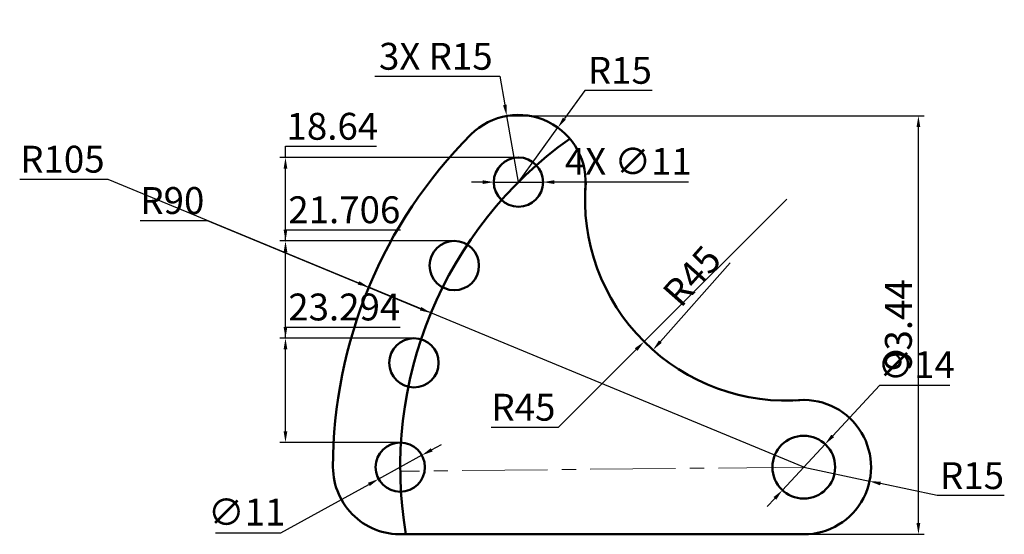
# Model space of a CAD drawing. Units: millimetres. Extents: x 68 to 288, y 29 to 144.
import ezdxf

# ---------------------------------------------------------------- set-up
doc = ezdxf.new("R2010")
doc.units = ezdxf.units.MM
doc.linetypes.add('CENTER2', pattern=[28.575, 19.05, -3.175, 3.175, -3.175])
for name, color, linetype, lineweight in [('M-CNTR', 4, 'CENTER2', 18), ('M-DIMS', 2, 'Continuous', 25), ('M-OUTL', 7, 'Continuous', 50)]:
    doc.layers.add(name, color=color, linetype=linetype, lineweight=lineweight)
doc.styles.get("Standard").update_dxf_attribs({"font": 'arial.ttf'})
doc.dimstyles.new('ISO-25', dxfattribs={"dimtxt": 6, "dimasz": 2.5, "dimexe": 1.25, "dimexo": 0.625, "dimtad": 1, "dimtoh": 1, "dimdec": 0, "dimtxsty": 'Standard', "dimcen": 2.5, "dimadec": 0, "dimazin": 0, "dimtfac": 1, "dimtdec": 0, "dimtmove": 0, "dimatfit": 3, "dimfxl": 1, "dimarcsym": 0})

# ---------------------------------------------------------------- blocks, each defined once
blk = doc.blocks.new('*U1')
blk.add_circle((0, 0), 5.5)
blk = doc.blocks.new('*U2')
at = {"layer": 'M-OUTL', "color": 0, "linetype": 'ByBlock', "lineweight": -2, "transparency": 16777216}
for p, rotation in [((49.87, 107.45), 315.0000000000001), ((35.56, 88.81), 330.0000000000001), ((26.57, 67.1), 344.9999999999999)]:
    blk.add_blockref('*U1', p, dxfattribs=dict(at, rotation=rotation))
blk.add_blockref('*U1', (23.51, 43.81), dxfattribs=at)
blk = doc.blocks.new('*D3')
at = {"layer": 'Defpoints', "color": 0, "transparency": 16777216}
for p in [(239.43, 103.65), (209.58, 69.97)]:
    blk.add_point(p, dxfattribs=at)
at = {"layer": 'M-DIMS', "color": 0, "lineweight": -2, "transparency": 16777216}
blk.add_line((226.8, 89.4), (211.24, 71.84), dxfattribs=at)
at = {"layer": 'M-DIMS', "color": 0, "transparency": 16777216}
blk.add_solid([(210.93, 72.11), (211.55, 71.56), (209.58, 69.97)], dxfattribs=at)
at = {"layer": 'M-DIMS', "color": 0, "transparency": 16777216, "insert": (218.86, 85.98), "char_height": 6, "attachment_point": 5, "rotation": 48.4597}
blk.add_mtext('R45', dxfattribs=at)
blk = doc.blocks.new('*D4')
at = {"layer": 'Defpoints', "color": 0, "transparency": 16777216}
for p in [(247.98, 48.95), (238.47, 38.67)]:
    blk.add_point(p, dxfattribs=at)
at = {"layer": 'M-DIMS', "color": 0, "lineweight": -2, "transparency": 16777216}
for p, q in [((260.11, 62.06), (249.68, 50.78)), ((275.84, 62.06), (260.11, 62.06)), ((238.47, 38.67), (247.98, 48.95)), ((236.77, 36.84), (235.08, 35))]:
    blk.add_line(p, q, dxfattribs=at)
at = {"layer": 'M-DIMS', "color": 0, "transparency": 16777216}
for points in [[(249.37, 51.06), (249.98, 50.5), (247.98, 48.95)], [(236.47, 37.12), (237.08, 36.55), (238.47, 38.67)]]:
    blk.add_solid(points, dxfattribs=at)
at = {"layer": 'M-DIMS', "color": 0, "transparency": 16777216, "insert": (268.29, 65.92), "char_height": 6, "attachment_point": 5}
blk.add_mtext('∅14', dxfattribs=at)
blk = doc.blocks.new('*D5')
at = {"layer": 'Defpoints', "color": 0, "transparency": 16777216}
for p in [(243.23, 43.81), (257.89, 40.67)]:
    blk.add_point(p, dxfattribs=at)
at = {"layer": 'M-DIMS', "color": 0, "lineweight": -2, "transparency": 16777216}
for p, q in [((243.23, 43.81), (257.89, 40.67)), ((272.95, 37.45), (260.34, 40.15)), ((287.95, 37.45), (272.95, 37.45))]:
    blk.add_line(p, q, dxfattribs=at)
at = {"layer": 'M-DIMS', "color": 0, "transparency": 16777216}
blk.add_solid([(260.43, 40.56), (260.25, 39.74), (257.89, 40.67)], dxfattribs=at)
at = {"layer": 'M-DIMS', "color": 0, "transparency": 16777216, "insert": (280.76, 41.14), "char_height": 6, "attachment_point": 5}
blk.add_mtext('R15', dxfattribs=at)
blk = doc.blocks.new('*D6')
at = {"layer": 'Defpoints', "color": 0, "transparency": 16777216}
for p in [(158.04, 46.46), (148.41, 41.16)]:
    blk.add_point(p, dxfattribs=at)
at = {"layer": 'M-DIMS', "color": 0, "lineweight": -2, "transparency": 16777216}
for p, q in [((160.23, 47.67), (162.42, 48.87)), ((158.04, 46.46), (148.41, 41.16)), ((126.58, 29.14), (146.22, 39.95)), ((111.99, 29.14), (126.58, 29.14))]:
    blk.add_line(p, q, dxfattribs=at)
at = {"layer": 'M-DIMS', "color": 0, "transparency": 16777216}
for points in [[(160.03, 48.03), (160.43, 47.3), (158.04, 46.46)], [(146.02, 40.32), (146.42, 39.59), (148.41, 41.16)]]:
    blk.add_solid(points, dxfattribs=at)
at = {"layer": 'M-DIMS', "color": 0, "transparency": 16777216, "insert": (118.97, 32.99), "char_height": 6, "attachment_point": 5}
blk.add_mtext('∅11', dxfattribs=at)
blk = doc.blocks.new('*D7')
at = {"layer": 'Defpoints', "color": 0, "transparency": 16777216}
for p in [(188.37, 119.61), (179.59, 107.45)]:
    blk.add_point(p, dxfattribs=at)
at = {"layer": 'M-DIMS', "color": 0, "lineweight": -2, "transparency": 16777216}
for p, q in [((194.39, 127.94), (189.83, 121.63)), ((209.4, 127.94), (194.39, 127.94)), ((179.59, 107.45), (188.37, 119.61))]:
    blk.add_line(p, q, dxfattribs=at)
at = {"layer": 'M-DIMS', "color": 0, "transparency": 16777216}
blk.add_solid([(189.5, 121.88), (190.17, 121.39), (188.37, 119.61)], dxfattribs=at)
at = {"layer": 'M-DIMS', "color": 0, "transparency": 16777216, "insert": (202.21, 131.63), "char_height": 6, "attachment_point": 5}
blk.add_mtext('R15', dxfattribs=at)
blk = doc.blocks.new('*D8')
at = {"layer": 'Defpoints', "color": 0, "transparency": 16777216}
for p in [(127.63, 72.6), (156.29, 72.6), (153.23, 49.31)]:
    blk.add_point(p, dxfattribs=at)
at = {"layer": 'M-DIMS', "color": 0, "lineweight": -2, "transparency": 16777216}
for p, q in [((127.63, 72.6), (127.63, 75.1)), ((127.63, 75.1), (153.24, 75.1)), ((155.67, 72.6), (126.38, 72.6)), ((127.63, 51.81), (127.63, 70.1)), ((152.6, 49.31), (126.38, 49.31))]:
    blk.add_line(p, q, dxfattribs=at)
at = {"layer": 'M-DIMS', "color": 0, "transparency": 16777216}
for points in [[(127.21, 70.1), (128.04, 70.1), (127.63, 72.6)], [(127.21, 51.81), (128.04, 51.81), (127.63, 49.31)]]:
    blk.add_solid(points, dxfattribs=at)
at = {"layer": 'M-DIMS', "color": 0, "transparency": 16777216, "insert": (140.74, 78.79), "char_height": 6, "attachment_point": 5}
blk.add_mtext('23.294', dxfattribs=at)
blk = doc.blocks.new('*D9')
at = {"layer": 'Defpoints', "color": 0, "transparency": 16777216}
for p in [(127.63, 94.31), (165.28, 94.31), (156.29, 72.6)]:
    blk.add_point(p, dxfattribs=at)
at = {"layer": 'M-DIMS', "color": 0, "lineweight": -2, "transparency": 16777216}
for p, q in [((127.63, 94.31), (127.63, 96.81)), ((127.63, 96.81), (153.26, 96.81)), ((164.66, 94.31), (126.38, 94.31)), ((127.63, 75.1), (127.63, 91.81)), ((155.67, 72.6), (126.38, 72.6))]:
    blk.add_line(p, q, dxfattribs=at)
at = {"layer": 'M-DIMS', "color": 0, "transparency": 16777216}
for points in [[(127.21, 91.81), (128.04, 91.81), (127.63, 94.31)], [(127.21, 75.1), (128.04, 75.1), (127.63, 72.6)]]:
    blk.add_solid(points, dxfattribs=at)
at = {"layer": 'M-DIMS', "color": 0, "transparency": 16777216, "insert": (140.75, 100.5), "char_height": 6, "attachment_point": 5}
blk.add_mtext('21.706', dxfattribs=at)
blk = doc.blocks.new('*D10')
at = {"layer": 'Defpoints', "color": 0, "transparency": 16777216}
for p in [(127.63, 112.95), (179.59, 112.95), (165.28, 94.31)]:
    blk.add_point(p, dxfattribs=at)
at = {"layer": 'M-DIMS', "color": 0, "lineweight": -2, "transparency": 16777216}
for p, q in [((127.63, 112.95), (127.63, 115.45)), ((127.63, 115.45), (147.91, 115.45)), ((178.96, 112.95), (126.38, 112.95)), ((127.63, 96.81), (127.63, 110.45)), ((164.66, 94.31), (126.38, 94.31))]:
    blk.add_line(p, q, dxfattribs=at)
at = {"layer": 'M-DIMS', "color": 0, "transparency": 16777216}
for points in [[(127.21, 110.45), (128.04, 110.45), (127.63, 112.95)], [(127.21, 96.81), (128.04, 96.81), (127.63, 94.31)]]:
    blk.add_solid(points, dxfattribs=at)
at = {"layer": 'M-DIMS', "color": 0, "transparency": 16777216, "insert": (138.08, 119.14), "char_height": 6, "attachment_point": 5}
blk.add_mtext('18.64', dxfattribs=at)
blk = doc.blocks.new('*D11')
at = {"layer": 'Defpoints', "color": 0, "transparency": 16777216}
for p in [(177.13, 122.25), (268.8, 122.25), (243.23, 28.81)]:
    blk.add_point(p, dxfattribs=at)
at = {"layer": 'M-DIMS', "color": 0, "lineweight": -2, "transparency": 16777216}
for p, q in [((177.75, 122.25), (270.05, 122.25)), ((268.8, 31.31), (268.8, 119.75)), ((243.85, 28.81), (270.05, 28.81))]:
    blk.add_line(p, q, dxfattribs=at)
at = {"layer": 'M-DIMS', "color": 0, "transparency": 16777216}
for points in [[(268.38, 119.75), (269.21, 119.75), (268.8, 122.25)], [(268.38, 31.31), (269.21, 31.31), (268.8, 28.81)]]:
    blk.add_solid(points, dxfattribs=at)
at = {"layer": 'M-DIMS', "color": 0, "transparency": 16777216, "insert": (265.11, 75.53), "char_height": 6, "attachment_point": 5, "rotation": 90}
blk.add_mtext('93.44', dxfattribs=at)
blk = doc.blocks.new('*D12')
at = {"layer": 'Defpoints', "color": 0, "transparency": 16777216}
for p in [(146.22, 83.99), (243.23, 43.81)]:
    blk.add_point(p, dxfattribs=at)
at = {"layer": 'M-DIMS', "color": 0, "lineweight": -2, "transparency": 16777216}
for p, q in [((68.35, 108.1), (88.01, 108.1)), ((88.01, 108.1), (143.91, 84.95)), ((243.23, 43.81), (146.22, 83.99))]:
    blk.add_line(p, q, dxfattribs=at)
at = {"layer": 'M-DIMS', "color": 0, "transparency": 16777216}
blk.add_solid([(144.07, 85.33), (143.75, 84.56), (146.22, 83.99)], dxfattribs=at)
at = {"layer": 'M-DIMS', "color": 0, "transparency": 16777216, "insert": (77.87, 111.79), "char_height": 6, "attachment_point": 5}
blk.add_mtext('R105', dxfattribs=at)
blk = doc.blocks.new('*D13')
at = {"layer": 'Defpoints', "color": 0, "transparency": 16777216}
for p in [(160.07, 78.23), (243.23, 43.81)]:
    blk.add_point(p, dxfattribs=at)
at = {"layer": 'M-DIMS', "color": 0, "lineweight": -2, "transparency": 16777216}
for p, q in [((95.23, 98.88), (110.17, 98.88)), ((110.17, 98.88), (157.76, 79.18)), ((243.23, 43.81), (160.07, 78.23))]:
    blk.add_line(p, q, dxfattribs=at)
at = {"layer": 'M-DIMS', "color": 0, "transparency": 16777216}
blk.add_solid([(157.92, 79.57), (157.6, 78.8), (160.07, 78.23)], dxfattribs=at)
at = {"layer": 'M-DIMS', "color": 0, "transparency": 16777216, "insert": (102.39, 102.56), "char_height": 6, "attachment_point": 5}
blk.add_mtext('R90', dxfattribs=at)
blk = doc.blocks.new('*D14')
at = {"layer": 'Defpoints', "color": 0, "transparency": 16777216}
for p in [(239.43, 103.65), (207.61, 71.83)]:
    blk.add_point(p, dxfattribs=at)
at = {"layer": 'M-DIMS', "color": 0, "lineweight": -2, "transparency": 16777216}
for p, q in [((239.43, 103.65), (207.61, 71.83)), ((188.51, 52.74), (205.84, 70.06)), ((173.51, 52.74), (188.51, 52.74))]:
    blk.add_line(p, q, dxfattribs=at)
at = {"layer": 'M-DIMS', "color": 0, "transparency": 16777216}
blk.add_solid([(205.54, 70.36), (206.13, 69.77), (207.61, 71.83)], dxfattribs=at)
at = {"layer": 'M-DIMS', "color": 0, "transparency": 16777216, "insert": (180.7, 56.41), "char_height": 6, "attachment_point": 5}
blk.add_mtext('R45', dxfattribs=at)
blk = doc.blocks.new('*D15')
at = {"layer": 'Defpoints', "color": 0, "transparency": 16777216}
for p in [(176.98, 122.22), (179.59, 107.45)]:
    blk.add_point(p, dxfattribs=at)
at = {"layer": 'M-DIMS', "color": 0, "lineweight": -2, "transparency": 16777216}
for p, q in [((147.52, 131.08), (175.42, 131.08)), ((175.42, 131.08), (176.55, 124.68)), ((179.59, 107.45), (176.98, 122.22))]:
    blk.add_line(p, q, dxfattribs=at)
at = {"layer": 'M-DIMS', "color": 0, "transparency": 16777216}
blk.add_solid([(176.96, 124.76), (176.14, 124.61), (176.98, 122.22)], dxfattribs=at)
at = {"layer": 'M-DIMS', "color": 0, "transparency": 16777216, "insert": (161.16, 134.77), "char_height": 6, "attachment_point": 5}
blk.add_mtext('3X R15', dxfattribs=at)
blk = doc.blocks.new('*D16')
at = {"layer": 'Defpoints', "color": 0, "transparency": 16777216}
for p in [(174.09, 107.45), (185.09, 107.45)]:
    blk.add_point(p, dxfattribs=at)
at = {"layer": 'M-DIMS', "color": 0, "lineweight": -2, "transparency": 16777216}
for p, q in [((171.59, 107.45), (169.09, 107.45)), ((174.09, 107.45), (185.09, 107.45)), ((190.09, 107.45), (187.59, 107.45)), ((217.49, 107.45), (190.09, 107.45))]:
    blk.add_line(p, q, dxfattribs=at)
at = {"layer": 'M-DIMS', "color": 0, "transparency": 16777216}
for points in [[(171.59, 107.87), (171.59, 107.03), (174.09, 107.45)], [(187.59, 107.87), (187.59, 107.03), (185.09, 107.45)]]:
    blk.add_solid(points, dxfattribs=at)
at = {"layer": 'M-DIMS', "color": 0, "transparency": 16777216, "insert": (204.1, 111.31), "char_height": 6, "attachment_point": 5}
blk.add_mtext('4X ∅11', dxfattribs=at)

msp = doc.modelspace()

# ---------------------------------------------------------------- linework, layer by layer
at = {"layer": 'M-CNTR'}
msp.add_line((243.2259, 43.8093), (153.2306, 42.8892), dxfattribs=at)
at = {"layer": 'M-OUTL'}
for points in [[(194.4657, 105.5513, 0.71505833), (168.9797, 118.0555, 0.19891237), (138.2259, 43.8093, 0.43886623), (154.4759, 28.8615)], [(191.0398, 117.1347, 0.28747486), (154.4847, 28.8093), (243.2259, 28.8093, 1.06552444), (241.3282, 58.6888)]]:
    msp.add_lwpolyline(points, format="xyb", dxfattribs=at)
for centre, radius in [((179.5863, 107.4489), 5.5), ((243.2259, 43.8093), 7)]:
    msp.add_circle(centre, radius, dxfattribs=at)
msp.add_arc((239.4255, 103.6485), 45, 175.155444, 274.844556, dxfattribs=at)

# ---------------------------------------------------------------- block references
msp.add_blockref('*U2', (129.7195, 0), dxfattribs=at)

# ---------------------------------------------------------------- dimensions: what is measured, and where the dimension line sits
at = {"layer": 'M-DIMS'}
dim = msp.add_radius_dim(center=(179.5863, 107.4489), mpoint=(176.98, 122.2207), text='3X <>', dimstyle='ISO-25', override={"dimdec": 0, "dimlfac": 1, "dimrnd": 0, "dimzin": 0, "dimdsep": 46, "dimlunit": 2}, dxfattribs=at)
dim.commit()
dim.dimension.update_dxf_attribs({"geometry": '*D15', "text_midpoint": (161.1563, 131.0839), "dimtype": 164})
for center, mpoint, override, picture, middle in [((179.5863, 107.4489), (188.3708, 119.6075), {"dimclrd": 0, "dimclre": 0, "dimclrt": 0}, '*D7', (202.2068, 127.9399)), ((243.2259, 43.8093), (146.2186, 83.9912), {"dimdec": 0, "dimlfac": 1, "dimrnd": 0, "dimzin": 0, "dimdsep": 46, "dimlunit": 2}, '*D12', (77.8674, 108.1003)), ((243.2259, 43.8093), (160.0665, 78.2262), {"dimdec": 0, "dimlfac": 1, "dimrnd": 0, "dimzin": 0, "dimdsep": 46, "dimlunit": 2}, '*D13', (102.3877, 98.8763)), ((239.4255, 103.6485), (207.6057, 71.8287), {"dimdec": 0, "dimlfac": 1, "dimrnd": 0, "dimzin": 0, "dimdsep": 46, "dimlunit": 2}, '*D14', (180.6978, 52.7368)), ((239.4255, 103.6485), (209.5839, 69.9665), {"dimclrd": 0, "dimclre": 0, "dimclrt": 0}, '*D3', (221.615, 83.5459)), ((243.2259, 43.8093), (257.8942, 40.6724), {"dimclrd": 0, "dimclre": 0, "dimclrt": 0}, '*D5', (272.9479, 37.4532))]:
    dim = msp.add_radius_dim(center=center, mpoint=mpoint, dimstyle='ISO-25', override=override, dxfattribs=at)
    dim.commit()
    dim.dimension.update_dxf_attribs({"geometry": picture, "text_midpoint": middle, "dimtype": 164})
for base, p1, p2, override, picture, middle in [((127.6259, 112.9489), (165.2836, 94.3093), (179.5863, 112.9489), {"dimdec": 2, "dimlfac": 1, "dimrnd": 0, "dimzin": 0, "dimdsep": 46, "dimlunit": 2}, '*D10', (138.0796, 119.1373)), ((268.7957, 122.2461), (243.2259, 28.8093), (177.1278, 122.2461), {"dimdec": 2, "dimlfac": 1, "dimrnd": 0, "dimzin": 0, "dimdsep": 46, "dimlunit": 2}, '*D11', (265.1052, 75.5277)), ((127.6259, 94.3093), (156.2925, 72.603), (165.2836, 94.3093), {"dimdec": 3, "dimlfac": 1, "dimrnd": 0, "dimzin": 0, "dimdsep": 46, "dimlunit": 2}, '*D9', (140.7543, 100.4977)), ((127.6259, 72.603), (153.2259, 49.3093), (156.2925, 72.603), {"dimdec": 3, "dimlfac": 1, "dimrnd": 0, "dimzin": 0, "dimdsep": 46, "dimlunit": 2}, '*D8', (140.744, 78.7935))]:
    dim = msp.add_linear_dim(base=base, p1=p1, p2=p2, angle=90, dimstyle='ISO-25', override=override, dxfattribs=at)
    dim.commit()
    dim.dimension.update_dxf_attribs({"geometry": picture, "text_midpoint": middle})
dim = msp.add_diameter_dim_2p(p1=(174.0863, 107.4488), p2=(185.0863, 107.449), text='4X <>', dimstyle='ISO-25', override={"dimdec": 0, "dimlfac": 1, "dimrnd": 0, "dimzin": 0, "dimdsep": 46, "dimlunit": 2}, dxfattribs=at)
dim.commit()
dim.dimension.update_dxf_attribs({"geometry": '*D16', "text_midpoint": (190.0863, 107.4491), "dimtype": 163})
for p1, p2, picture, middle in [((238.4714, 38.6717), (247.9803, 48.9469), '*D4', (268.2888, 62.0591)), ((158.0437, 46.4624), (148.4081, 41.1562), '*D6', (118.9727, 29.1357))]:
    dim = msp.add_diameter_dim_2p(p1=p1, p2=p2, dimstyle='ISO-25', override={"dimclrd": 0, "dimclre": 0, "dimclrt": 0}, dxfattribs=at)
    dim.commit()
    dim.dimension.update_dxf_attribs({"geometry": picture, "text_midpoint": middle, "dimtype": 163})

doc.saveas('drawing.dxf')
